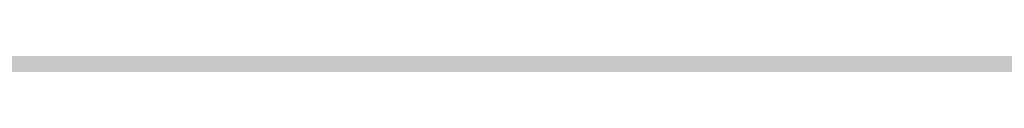
# Model space of a CAD drawing. Units: millimetres. Extents: x 0 to 2267, y 0 to 1823.
# Tile 171 of 256: x 1833.606 to 1838.83, y 1127.422 to 1127.431. Entities that reach past the tile are written whole.
import ezdxf

# ---------------------------------------------------------------- set-up
doc = ezdxf.new("R2010")
doc.units = ezdxf.units.MM
doc.header["$MEASUREMENT"] = 0
doc.layers.add('M-HATC', color=252, linetype='Continuous', lineweight=18)

msp = doc.modelspace()

# ---------------------------------------------------------------- hatches: boundary and pattern name
at = {"layer": 'M-HATC'}
h = msp.add_hatch(color=256, dxfattribs=at)
h.dxf.hatch_style = 1
h.paths.add_polyline_path([(2055.771, 1603.062), (1381.0868, 1603.062), (1381.0868, 1598.062), (2055.771, 1598.062)])
h.paths.add_polyline_path([(2055.771, 1598.062), (1381.0868, 1598.062), (1381.0868, 1593.062), (2055.771, 1593.062)])
h.paths.add_polyline_path([(2051.3074, 1536.7609), (1385.5504, 1536.7609), (1385.5504, 1526.7609), (1387.5504, 1526.7609), (1388.5366, 1525.0528), (1385.3319, 1521.2335), (1385.3319, 1521.2226), (2050.2542, 1522.7491), (2048.3212, 1525.0528), (2049.3074, 1526.7609), (2051.3074, 1526.7609)])
edge = h.paths.add_edge_path()
edge.add_arc((1847.5345, 1379.1492), 135, 222.603061, 222.890851, ccw=False)
edge.add_line((1748.1663, 1287.7656), (1683.0921, 1287.7656))
edge.add_arc((1583.7239, 1379.1492), 135, 317.109149, 317.396939, ccw=False)
edge.add_arc((1678.9686, 1290.6707), 5, 222.8909, 317.1091, ccw=False)
edge.add_arc((1774.2133, 1379.1492), 135, 222.603061, 222.890851, ccw=False)
edge.add_line((1674.8451, 1287.7656), (1609.7709, 1287.7656))
edge.add_arc((1510.4027, 1379.1492), 135, 317.109149, 317.396939, ccw=False)
edge.add_arc((1605.6474, 1290.6707), 5, 222.8909, 317.1091, ccw=False)
edge.add_arc((1700.8921, 1379.1492), 135, 222.603061, 222.890851, ccw=False)
edge.add_line((1601.5239, 1287.7656), (1536.4497, 1287.7656))
edge.add_arc((1437.0815, 1379.1492), 135, 317.109149, 317.396939, ccw=False)
edge.add_arc((1532.3262, 1290.6707), 5, 222.8909, 317.1091, ccw=False)
edge.add_arc((1627.5709, 1379.1492), 135, 222.603061, 222.890851, ccw=False)
edge.add_line((1528.2027, 1287.7656), (1505.9289, 1287.7656))
edge.add_spline(control_points=[(1505.9289, 1287.7656), (1504.2622, 1287.7656), (1504.2622, 1282.7656), (1505.9289, 1282.7656)], knot_values=[0, 0, 0, 0, 5, 5, 5, 5], degree=3, periodic=0)
edge.add_line((1505.9289, 1282.7656), (1930.9289, 1282.7656))
edge.add_spline(control_points=[(1930.9289, 1282.7656), (1932.5956, 1282.7656), (1932.5956, 1287.7656), (1930.9289, 1287.7656)], knot_values=[0, 0, 0, 0, 5, 5, 5, 5], degree=3, periodic=0)
edge.add_line((1930.9289, 1287.7656), (1903.0557, 1287.7656))
edge.add_arc((1803.6875, 1379.1492), 135, 317.109149, 317.396939, ccw=False)
edge.add_arc((1898.9322, 1290.6707), 5, 222.8909, 317.1091, ccw=False)
edge.add_arc((1994.1769, 1379.1492), 135, 222.603061, 222.890851, ccw=False)
edge.add_line((1894.8087, 1287.7656), (1829.7345, 1287.7656))
edge.add_arc((1730.3663, 1379.1492), 135, 317.109149, 317.396939, ccw=False)
edge.add_arc((1825.611, 1290.6707), 5, 222.8909, 317.1091, ccw=False)
edge.add_arc((1920.8557, 1379.1492), 135, 222.603061, 222.890851, ccw=False)
edge.add_line((1821.4875, 1287.7656), (1756.4133, 1287.7656))
edge.add_arc((1657.0451, 1379.1492), 135, 317.109149, 317.396939, ccw=False)
edge.add_arc((1752.2898, 1290.6707), 5, 222.8909, 317.1091, ccw=False)
edge = h.paths.add_edge_path()
edge.add_spline(control_points=[(1843.4289, 1227.2475), (1845.0956, 1227.2475), (1845.0956, 1232.2475), (1843.4289, 1232.2475)], knot_values=[0, 0, 0, 0, 5, 5, 5, 5], degree=3, periodic=0)
edge.add_line((1843.4289, 1232.2475), (1593.4289, 1232.2475))
edge.add_spline(control_points=[(1593.4289, 1232.2475), (1591.7622, 1232.2475), (1591.7622, 1227.2475), (1593.4289, 1227.2475)], knot_values=[0, 0, 0, 0, 5, 5, 5, 5], degree=3, periodic=0)
edge.add_line((1593.4289, 1227.2475), (1843.4289, 1227.2475))
h.paths.add_polyline_path([(1905.9289, 1127.4171), (1530.9289, 1127.4171, 0.414214), (1520.9289, 1117.4171), (1530.9289, 1117.4171), (1915.9289, 1117.4171, 0.414214)])
edge = h.paths.add_edge_path()
edge.add_arc((1397.0858, 1498.4078), 12.7299, 90.78215, 190.87871, ccw=False)
edge.add_line((1396.912, 1511.1365), (1428.0097, 1511.3488))
edge.add_line((1428.0097, 1511.3488), (1433.0097, 1511.3488))
edge.add_line((1433.0097, 1511.3488), (1434.439, 1511.3488))
edge.add_arc((1419.474, 1498.0804), 20, 41.561, 74.08211)
edge.add_line((1424.9592, 1517.3135), (1399.9351, 1517.2561))
edge.add_spline(control_points=[(1399.9307, 1517.2561), (1399.884, 1517.2131), (1399.8328, 1517.1689), (1399.7774, 1517.1236)], knot_values=[11.567499, 11.567499, 11.567499, 11.567499, 11.814249, 11.814249, 11.814249, 11.814249], degree=3, periodic=0)
edge.add_spline(control_points=[(1399.6328, 1517.0099), (1399.5831, 1516.9721), (1399.5307, 1516.9338), (1399.4759, 1516.8947)], knot_values=[11.167718, 11.167718, 11.167718, 11.167718, 11.365188, 11.365188, 11.365188, 11.365188], degree=3, periodic=0)
edge.add_spline(control_points=[(1399.3398, 1516.8001), (1399.1514, 1516.6719), (1398.9384, 1516.5377), (1398.704, 1516.3994)], knot_values=[10.376405, 10.376405, 10.376405, 10.376405, 11.00994, 11.00994, 11.00994, 11.00994], degree=3, periodic=0)
edge.add_spline(control_points=[(1398.6572, 1516.3719), (1398.5789, 1516.326), (1398.4983, 1516.2797), (1398.4155, 1516.2331)], knot_values=[10.125175, 10.125175, 10.125175, 10.125175, 10.334406, 10.334406, 10.334406, 10.334406], degree=3, periodic=0)
edge.add_spline(control_points=[(1398.2642, 1516.1487), (1398.196, 1516.1111), (1398.1263, 1516.0732), (1398.0555, 1516.0351)], knot_values=[9.832246, 9.832246, 9.832246, 9.832246, 9.999658, 9.999658, 9.999658, 9.999658], degree=3, periodic=0)
edge.add_spline(control_points=[(1397.9987, 1516.0048), (1397.7312, 1515.8621), (1397.446, 1515.7171), (1397.1466, 1515.5714)], knot_values=[9.161808, 9.161808, 9.161808, 9.161808, 9.787769, 9.787769, 9.787769, 9.787769], degree=3, periodic=0)
edge.add_spline(control_points=[(1397.1466, 1515.5714), (1396.8418, 1515.423), (1396.5222, 1515.274), (1396.1914, 1515.1262)], knot_values=[8.524455, 8.524455, 8.524455, 8.524455, 9.161808, 9.161808, 9.161808, 9.161808], degree=3, periodic=0)
edge.add_spline(control_points=[(1396.0777, 1515.0756), (1395.9854, 1515.0348), (1395.8922, 1514.994), (1395.7983, 1514.9534)], knot_values=[8.275193, 8.275193, 8.275193, 8.275193, 8.451726, 8.451726, 8.451726, 8.451726], degree=3, periodic=0)
edge.add_spline(control_points=[(1395.6018, 1514.8691), (1395.4997, 1514.8257), (1395.3968, 1514.7824), (1395.2932, 1514.7394)], knot_values=[7.962917, 7.962917, 7.962917, 7.962917, 8.152764, 8.152764, 8.152764, 8.152764], degree=3, periodic=0)
edge.add_spline(control_points=[(1395.2116, 1514.7057), (1394.8278, 1514.5475), (1394.4345, 1514.3929), (1394.0364, 1514.2442)], knot_values=[7.21254, 7.21254, 7.21254, 7.21254, 7.913148, 7.913148, 7.913148, 7.913148], degree=3, periodic=0)
edge.add_spline(control_points=[(1394.0364, 1514.2442), (1393.7076, 1514.1214), (1393.3754, 1514.0027), (1393.0427, 1513.8895)], knot_values=[6.633733, 6.633733, 6.633733, 6.633733, 7.21254, 7.21254, 7.21254, 7.21254], degree=3, periodic=0)
edge.add_spline(control_points=[(1392.8214, 1513.815), (1392.7198, 1513.7812), (1392.6181, 1513.7479), (1392.5166, 1513.7152)], knot_values=[6.328796, 6.328796, 6.328796, 6.328796, 6.505493, 6.505493, 6.505493, 6.505493], degree=3, periodic=0)
edge.add_spline(control_points=[(1392.5166, 1513.7152), (1392.3187, 1513.6515), (1392.1212, 1513.59), (1391.9244, 1513.531)], knot_values=[5.984605, 5.984605, 5.984605, 5.984605, 6.328796, 6.328796, 6.328796, 6.328796], degree=3, periodic=0)
edge.add_spline(control_points=[(1391.7915, 1513.4915), (1391.3122, 1513.3501), (1390.8384, 1513.2239), (1390.3784, 1513.1171)], knot_values=[5.066697, 5.066697, 5.066697, 5.066697, 5.907055, 5.907055, 5.907055, 5.907055], degree=3, periodic=0)
edge.add_spline(control_points=[(1390.3784, 1513.1171), (1390.1797, 1513.071), (1389.9836, 1513.0284), (1389.7907, 1512.9899)], knot_values=[4.70367, 4.70367, 4.70367, 4.70367, 5.066695, 5.066695, 5.066695, 5.066695], degree=3, periodic=0)
edge.add_spline(control_points=[(1389.422, 1512.9204), (1389.2459, 1512.8892), (1389.0729, 1512.8617), (1388.9036, 1512.8381)], knot_values=[4.130571, 4.130571, 4.130571, 4.130571, 4.469816, 4.469816, 4.469816, 4.469816], degree=3, periodic=0)
edge.add_spline(control_points=[(1388.9036, 1512.8381), (1388.591, 1512.7946), (1388.2911, 1512.7644), (1388.0071, 1512.7494)], knot_values=[3.504031, 3.504031, 3.504031, 3.504031, 4.130571, 4.130571, 4.130571, 4.130571], degree=3, periodic=0)
edge.add_spline(control_points=[(1387.9356, 1512.7459), (1387.8538, 1512.7423), (1387.7733, 1512.74), (1387.6944, 1512.739)], knot_values=[3.268866, 3.268866, 3.268866, 3.268866, 3.451164, 3.451164, 3.451164, 3.451164], degree=3, periodic=0)
edge.add_spline(control_points=[(1387.3351, 1512.7443), (1387.2076, 1512.7499), (1387.0847, 1512.7597), (1386.967, 1512.7739)], knot_values=[2.670686, 2.670686, 2.670686, 2.670686, 2.984, 2.984, 2.984, 2.984], degree=3, periodic=0)
edge.add_spline(control_points=[(1386.8327, 1512.7922), (1386.8209, 1512.7941), (1386.8092, 1512.7959), (1386.7975, 1512.7979)], knot_values=[2.516981, 2.516981, 2.516981, 2.516981, 2.549528, 2.549528, 2.549528, 2.549528], degree=3, periodic=0)
edge.add_spline(control_points=[(1386.4526, 1512.8735), (1386.4257, 1512.881), (1386.3993, 1512.889), (1386.3733, 1512.8972)], knot_values=[2.095869, 2.095869, 2.095869, 2.095869, 2.17941, 2.17941, 2.17941, 2.17941], degree=3, periodic=0)
edge.add_spline(control_points=[(1386.0691, 1513.0189), (1386.0634, 1513.0217), (1386.0577, 1513.0246), (1386.052, 1513.0275)], knot_values=[1.72453, 1.72453, 1.72453, 1.72453, 1.745933, 1.745933, 1.745933, 1.745933], degree=3, periodic=0)
edge.add_arc((1399.474, 1498.0804), 20, 131.82432, 180)
edge.add_arc((1630.3336, 1505.5484), 250.9708, 181.705176, 236.427975)
edge.add_arc((1605.3399, 1483.3044), 218.7822, 238.660829, 243.34961)
edge.add_arc((1647.0911, 1510.3592), 262.8986, 183.129836, 237.853442, ccw=False)
h.paths.add_polyline_path([(1406.5369, 1391.9644, 0.149382), (1491.5506, 1296.4418, -0.129517)], flags=17)
edge = h.paths.add_edge_path()
edge.add_arc((2037.3838, 1498.0804), 20, 0, 48.26587)
edge.add_spline(control_points=[(2050.6973, 1513.0052), (2050.6512, 1512.9847), (2050.6034, 1512.9655), (2050.5539, 1512.9477)], knot_values=[1.835652, 1.835652, 1.835652, 1.835652, 2.000781, 2.000781, 2.000781, 2.000781], degree=3, periodic=0)
edge.add_spline(control_points=[(2050.4616, 1512.9166), (2050.479, 1512.9221), (2050.4963, 1512.9277), (2050.5133, 1512.9335)], knot_values=[2.045477, 2.045477, 2.045477, 2.045477, 2.101389, 2.101389, 2.101389, 2.101389], degree=3, periodic=0)
edge.add_spline(control_points=[(2050.129, 1512.8342), (2050.1984, 1512.8473), (2050.2657, 1512.8623), (2050.3308, 1512.8792)], knot_values=[2.237629, 2.237629, 2.237629, 2.237629, 2.435841, 2.435841, 2.435841, 2.435841], degree=3, periodic=0)
edge.add_spline(control_points=[(2050.0946, 1512.8278), (2050.1061, 1512.8299), (2050.1176, 1512.832), (2050.129, 1512.8342)], knot_values=[2.435841, 2.435841, 2.435841, 2.435841, 2.468321, 2.468321, 2.468321, 2.468321], degree=3, periodic=0)
edge.add_spline(control_points=[(2049.7843, 1512.7851), (2049.8552, 1512.7922), (2049.9243, 1512.8008), (2049.9917, 1512.8109)], knot_values=[2.563852, 2.563852, 2.563852, 2.563852, 2.748541, 2.748541, 2.748541, 2.748541], degree=3, periodic=0)
edge.add_spline(control_points=[(2049.4052, 1512.7617), (2049.5364, 1512.7653), (2049.6629, 1512.773), (2049.7843, 1512.7851)], knot_values=[2.748541, 2.748541, 2.748541, 2.748541, 3.064882, 3.064882, 3.064882, 3.064882], degree=3, periodic=0)
edge.add_spline(control_points=[(2049.1698, 1512.7597), (2049.2336, 1512.7591), (2049.2965, 1512.7594), (2049.3584, 1512.7606)], knot_values=[3.102309, 3.102309, 3.102309, 3.102309, 3.2503, 3.2503, 3.2503, 3.2503], degree=3, periodic=0)
edge.add_spline(control_points=[(2048.8573, 1512.7691), (2048.9638, 1512.7638), (2049.068, 1512.7606), (2049.1698, 1512.7597)], knot_values=[3.2503, 3.2503, 3.2503, 3.2503, 3.486069, 3.486069, 3.486069, 3.486069], degree=3, periodic=0)
edge.add_spline(control_points=[(2048.6924, 1512.7789), (2048.3729, 1512.8009), (2048.0345, 1512.8411), (2047.6817, 1512.897)], knot_values=[3.606429, 3.606429, 3.606429, 3.606429, 4.2989, 4.2989, 4.2989, 4.2989], degree=3, periodic=0)
edge.add_spline(control_points=[(2047.6817, 1512.897), (2047.5458, 1512.9185), (2047.4077, 1512.9424), (2047.2678, 1512.9685)], knot_values=[4.2989, 4.2989, 4.2989, 4.2989, 4.565769, 4.565769, 4.565769, 4.565769], degree=3, periodic=0)
edge.add_spline(control_points=[(2047.2678, 1512.9685), (2047.1449, 1512.9914), (2047.0207, 1513.016), (2046.8951, 1513.0422)], knot_values=[4.565769, 4.565769, 4.565769, 4.565769, 4.799971, 4.799971, 4.799971, 4.799971], degree=3, periodic=0)
edge.add_spline(control_points=[(2046.8951, 1513.0422), (2046.5286, 1513.1188), (2046.1513, 1513.209), (2045.7676, 1513.3107)], knot_values=[4.799971, 4.799971, 4.799971, 4.799971, 5.483718, 5.483718, 5.483718, 5.483718], degree=3, periodic=0)
edge.add_spline(control_points=[(2045.7676, 1513.3107), (2045.3724, 1513.4154), (2044.9704, 1513.5322), (2044.5662, 1513.6588)], knot_values=[5.483718, 5.483718, 5.483718, 5.483718, 6.187866, 6.187866, 6.187866, 6.187866], degree=3, periodic=0)
edge.add_spline(control_points=[(2044.5662, 1513.6588), (2044.4149, 1513.7061), (2044.2633, 1513.7549), (2044.1116, 1513.8048)], knot_values=[6.187866, 6.187866, 6.187866, 6.187866, 6.451551, 6.451551, 6.451551, 6.451551], degree=3, periodic=0)
edge.add_spline(control_points=[(2044.1116, 1513.8048), (2043.9967, 1513.8427), (2043.8817, 1513.8813), (2043.7668, 1513.9205)], knot_values=[6.451551, 6.451551, 6.451551, 6.451551, 6.651434, 6.651434, 6.651434, 6.651434], degree=3, periodic=0)
edge.add_spline(control_points=[(2043.7668, 1513.9205), (2043.3716, 1514.0554), (2042.9774, 1514.1979), (2042.5886, 1514.3458)], knot_values=[6.651434, 6.651434, 6.651434, 6.651434, 7.338879, 7.338879, 7.338879, 7.338879], degree=3, periodic=0)
edge.add_spline(control_points=[(2042.5886, 1514.3458), (2042.1643, 1514.5071), (2041.7465, 1514.6749), (2041.3409, 1514.846)], knot_values=[7.338879, 7.338879, 7.338879, 7.338879, 8.089209, 8.089209, 8.089209, 8.089209], degree=3, periodic=0)
edge.add_spline(control_points=[(2041.3409, 1514.846), (2041.1028, 1514.9465), (2040.869, 1515.0481), (2040.6405, 1515.1502)], knot_values=[8.089209, 8.089209, 8.089209, 8.089209, 8.529587, 8.529587, 8.529587, 8.529587], degree=3, periodic=0)
edge.add_spline(control_points=[(2040.51, 1515.2089), (2040.0824, 1515.4022), (2039.6747, 1515.5971), (2039.295, 1515.7894)], knot_values=[8.613818, 8.613818, 8.613818, 8.613818, 9.44571, 9.44571, 9.44571, 9.44571], degree=3, periodic=0)
edge.add_spline(control_points=[(2039.295, 1515.7894), (2039.0618, 1515.9075), (2038.8391, 1516.0246), (2038.6288, 1516.1398)], knot_values=[9.44571, 9.44571, 9.44571, 9.44571, 9.956404, 9.956404, 9.956404, 9.956404], degree=3, periodic=0)
edge.add_spline(control_points=[(2038.6288, 1516.1398), (2038.5187, 1516.2001), (2038.4121, 1516.2598), (2038.309, 1516.3189)], knot_values=[9.956404, 9.956404, 9.956404, 9.956404, 10.223542, 10.223542, 10.223542, 10.223542], degree=3, periodic=0)
edge.add_spline(control_points=[(2038.309, 1516.3189), (2038.2138, 1516.3735), (2038.1216, 1516.4276), (2038.0328, 1516.481)], knot_values=[10.223542, 10.223542, 10.223542, 10.223542, 10.47051, 10.47051, 10.47051, 10.47051], degree=3, periodic=0)
edge.add_spline(control_points=[(2038.0328, 1516.481), (2037.7855, 1516.6296), (2037.5639, 1516.773), (2037.3722, 1516.909)], knot_values=[10.47051, 10.47051, 10.47051, 10.47051, 11.15767, 11.15767, 11.15767, 11.15767], degree=3, periodic=0)
edge.add_spline(control_points=[(2037.3722, 1516.909), (2037.2789, 1516.9752), (2037.1927, 1517.0396), (2037.1142, 1517.102)], knot_values=[11.15767, 11.15767, 11.15767, 11.15767, 11.49227, 11.49227, 11.49227, 11.49227], degree=3, periodic=0)
edge.add_spline(control_points=[(2036.8564, 1517.3259), (2036.9148, 1517.2692), (2036.9814, 1517.2103), (2037.0557, 1517.1492)], knot_values=[11.577341, 11.577341, 11.577341, 11.577341, 11.91035, 11.91035, 11.91035, 11.91035], degree=3, periodic=0)
edge.add_spline(control_points=[(2036.8074, 1517.3748), (2036.823, 1517.3587), (2036.8393, 1517.3424), (2036.8564, 1517.3259)], knot_values=[11.91035, 11.91035, 11.91035, 11.91035, 12.007402, 12.007402, 12.007402, 12.007402], degree=3, periodic=0)
edge.add_spline(control_points=[(2036.7017, 1517.494), (2036.7104, 1517.483), (2036.7196, 1517.4719), (2036.7291, 1517.4606)], knot_values=[12.184155, 12.184155, 12.184155, 12.184155, 12.255409, 12.255409, 12.255409, 12.255409], degree=3, periodic=0)
edge.add_spline(control_points=[(2036.6159, 1517.6205), (2036.62, 1517.613), (2036.6243, 1517.6055), (2036.6289, 1517.5979)], knot_values=[12.487913, 12.487913, 12.487913, 12.487913, 12.541035, 12.541035, 12.541035, 12.541035], degree=3, periodic=0)
edge.add_spline(control_points=[(2036.5635, 1517.786), (2036.5637, 1517.7794), (2036.5642, 1517.7726), (2036.565, 1517.7658)], knot_values=[12.911761, 12.911761, 12.911761, 12.911761, 12.968286, 12.968286, 12.968286, 12.968286], degree=3, periodic=0)
edge.add_spline(control_points=[(2036.6166, 1517.9304), (2036.6125, 1517.9259), (2036.6086, 1517.9212), (2036.6049, 1517.9165)], knot_values=[13.382527, 13.382527, 13.382527, 13.382527, 13.433791, 13.433791, 13.433791, 13.433791], degree=3, periodic=0)
edge.add_spline(control_points=[(2036.749, 1518.017), (2036.7361, 1518.0116), (2036.7239, 1518.006), (2036.7124, 1518.0002)], knot_values=[13.726299, 13.726299, 13.726299, 13.726299, 13.809928, 13.809928, 13.809928, 13.809928], degree=3, periodic=0)
edge.add_spline(control_points=[(2036.8604, 1518.0528), (2036.8386, 1518.0474), (2036.8181, 1518.0416), (2036.7988, 1518.0353)], knot_values=[13.910887, 13.910887, 13.910887, 13.910887, 14.02153, 14.02153, 14.02153, 14.02153], degree=3, periodic=0)
edge.add_line((2036.9639, 1518.0804), (2032.3838, 1518.0804))
edge.add_line((2032.3838, 1518.0804), (2027.3838, 1518.0804))
edge.add_line((2027.3838, 1518.0804), (2022.3838, 1518.0804))
edge.add_line((2022.3838, 1518.0804), (2017.3838, 1518.0804))
edge.add_arc((2017.3838, 1498.0804), 20, 90, 138.439)
edge.add_line((2002.4188, 1511.3488), (2003.8481, 1511.3488))
edge.add_line((2003.8481, 1511.3488), (2008.8481, 1511.3488))
edge.add_line((2008.8481, 1511.3488), (2039.772, 1511.1377))
edge.add_arc((2039.772, 1498.4078), 12.7299, -10.87871, 90, ccw=False)
edge.add_arc((1789.7668, 1510.3592), 262.8986, 302.146558, 356.870164, ccw=False)
edge.add_arc((1831.5179, 1483.3044), 218.7822, 296.65039, 301.339171)
edge.add_arc((1806.5242, 1505.5484), 250.9708, 303.572025, 358.294824)
h.paths.add_polyline_path([(2030.321, 1391.9644, -0.129517), (1945.3072, 1296.4418, 0.149382)], flags=17)
edge = h.paths.add_edge_path()
edge.add_spline(control_points=[(2037.2464, 1518.0821), (2037.2898, 1518.081), (2037.3355, 1518.0804), (2037.3838, 1518.0804)], knot_values=[0.000012, 0.000012, 0.000012, 0.000012, 0.144754, 0.144754, 0.144754, 0.144754], degree=3, periodic=0)
edge.add_line((2037.3357, 1518.0804), (2037.0096, 1518.0804))
edge.add_spline(control_points=[(2037.0096, 1518.0804), (2036.9822, 1518.0768), (2036.956, 1518.0727), (2036.9312, 1518.0681)], knot_values=[14.13465, 14.13465, 14.13465, 14.13465, 14.247197, 14.247197, 14.247197, 14.247197], degree=3, periodic=0)
edge.add_spline(control_points=[(2036.9312, 1518.0681), (2036.9276, 1518.0674), (2036.9241, 1518.0667), (2036.9205, 1518.0661)], knot_values=[14.118315, 14.118315, 14.118315, 14.118315, 14.13465, 14.13465, 14.13465, 14.13465], degree=3, periodic=0)
edge.add_spline(control_points=[(2036.9205, 1518.0661), (2036.9118, 1518.0644), (2036.9032, 1518.0626), (2036.8948, 1518.0608)], knot_values=[14.078086, 14.078086, 14.078086, 14.078086, 14.118315, 14.118315, 14.118315, 14.118315], degree=3, periodic=0)
edge.add_spline(control_points=[(2036.8948, 1518.0608), (2036.883, 1518.0583), (2036.8716, 1518.0556), (2036.8604, 1518.0528)], knot_values=[14.02153, 14.02153, 14.02153, 14.02153, 14.078086, 14.078086, 14.078086, 14.078086], degree=3, periodic=0)
edge.add_spline(control_points=[(2036.8604, 1518.0528), (2036.8386, 1518.0474), (2036.8181, 1518.0416), (2036.7988, 1518.0353)], knot_values=[13.910887, 13.910887, 13.910887, 13.910887, 14.02153, 14.02153, 14.02153, 14.02153], degree=3, periodic=0)
edge.add_spline(control_points=[(2036.7988, 1518.0353), (2036.7981, 1518.035), (2036.7974, 1518.0348), (2036.7967, 1518.0346)], knot_values=[13.906906, 13.906906, 13.906906, 13.906906, 13.910887, 13.910887, 13.910887, 13.910887], degree=3, periodic=0)
edge.add_spline(control_points=[(2036.7967, 1518.0346), (2036.7882, 1518.0318), (2036.7799, 1518.0289), (2036.7719, 1518.0259)], knot_values=[13.857826, 13.857826, 13.857826, 13.857826, 13.906906, 13.906906, 13.906906, 13.906906], degree=3, periodic=0)
edge.add_spline(control_points=[(2036.7719, 1518.0259), (2036.764, 1518.023), (2036.7564, 1518.02), (2036.749, 1518.017)], knot_values=[13.809928, 13.809928, 13.809928, 13.809928, 13.857826, 13.857826, 13.857826, 13.857826], degree=3, periodic=0)
edge.add_spline(control_points=[(2036.749, 1518.017), (2036.7361, 1518.0116), (2036.7239, 1518.006), (2036.7124, 1518.0002)], knot_values=[13.726299, 13.726299, 13.726299, 13.726299, 13.809928, 13.809928, 13.809928, 13.809928], degree=3, periodic=0)
edge.add_spline(control_points=[(2036.7124, 1518.0002), (2036.7121, 1518), (2036.7118, 1517.9999), (2036.7115, 1517.9997)], knot_values=[13.723993, 13.723993, 13.723993, 13.723993, 13.726299, 13.726299, 13.726299, 13.726299], degree=3, periodic=0)
edge.add_spline(control_points=[(2036.7115, 1517.9997), (2036.7063, 1517.9971), (2036.7013, 1517.9944), (2036.6965, 1517.9917)], knot_values=[13.686536, 13.686536, 13.686536, 13.686536, 13.723993, 13.723993, 13.723993, 13.723993], degree=3, periodic=0)
edge.add_spline(control_points=[(2036.6965, 1517.9917), (2036.6919, 1517.9891), (2036.6874, 1517.9865), (2036.6831, 1517.9839)], knot_values=[13.651251, 13.651251, 13.651251, 13.651251, 13.686536, 13.686536, 13.686536, 13.686536], degree=3, periodic=0)
edge.add_spline(control_points=[(2036.6831, 1517.9839), (2036.6764, 1517.9798), (2036.67, 1517.9757), (2036.6639, 1517.9714)], knot_values=[13.596804, 13.596804, 13.596804, 13.596804, 13.651251, 13.651251, 13.651251, 13.651251], degree=3, periodic=0)
edge.add_spline(control_points=[(2036.6639, 1517.9714), (2036.6636, 1517.9712), (2036.6633, 1517.9709), (2036.6629, 1517.9707)], knot_values=[13.593956, 13.593956, 13.593956, 13.593956, 13.596804, 13.596804, 13.596804, 13.596804], degree=3, periodic=0)
edge.add_spline(control_points=[(2036.6629, 1517.9707), (2036.6603, 1517.9689), (2036.6577, 1517.967), (2036.6552, 1517.9651)], knot_values=[13.570322, 13.570322, 13.570322, 13.570322, 13.593956, 13.593956, 13.593956, 13.593956], degree=3, periodic=0)
edge.add_spline(control_points=[(2036.6552, 1517.9651), (2036.6525, 1517.9631), (2036.6499, 1517.9611), (2036.6474, 1517.9591)], knot_values=[13.545477, 13.545477, 13.545477, 13.545477, 13.570322, 13.570322, 13.570322, 13.570322], degree=3, periodic=0)
edge.add_spline(control_points=[(2036.6474, 1517.9591), (2036.6472, 1517.9589), (2036.6471, 1517.9588), (2036.6469, 1517.9587)], knot_values=[13.543931, 13.543931, 13.543931, 13.543931, 13.545477, 13.545477, 13.545477, 13.545477], degree=3, periodic=0)
edge.add_spline(control_points=[(2036.6469, 1517.9587), (2036.6412, 1517.9541), (2036.6358, 1517.9494), (2036.6307, 1517.9447)], knot_values=[13.488237, 13.488237, 13.488237, 13.488237, 13.543931, 13.543931, 13.543931, 13.543931], degree=3, periodic=0)
edge.add_spline(control_points=[(2036.6307, 1517.9447), (2036.6282, 1517.9423), (2036.6257, 1517.9399), (2036.6233, 1517.9374)], knot_values=[13.460307, 13.460307, 13.460307, 13.460307, 13.488237, 13.488237, 13.488237, 13.488237], degree=3, periodic=0)
edge.add_spline(control_points=[(2036.6233, 1517.9374), (2036.6215, 1517.9356), (2036.6198, 1517.9338), (2036.6181, 1517.932)], knot_values=[13.439712, 13.439712, 13.439712, 13.439712, 13.460307, 13.460307, 13.460307, 13.460307], degree=3, periodic=0)
edge.add_spline(control_points=[(2036.6181, 1517.932), (2036.6176, 1517.9315), (2036.6171, 1517.9309), (2036.6166, 1517.9304)], knot_values=[13.433791, 13.433791, 13.433791, 13.433791, 13.439712, 13.439712, 13.439712, 13.439712], degree=3, periodic=0)
edge.add_spline(control_points=[(2036.6166, 1517.9304), (2036.6125, 1517.9259), (2036.6086, 1517.9212), (2036.6049, 1517.9165)], knot_values=[13.382527, 13.382527, 13.382527, 13.382527, 13.433791, 13.433791, 13.433791, 13.433791], degree=3, periodic=0)
edge.add_spline(control_points=[(2036.6049, 1517.9165), (2036.6026, 1517.9135), (2036.6004, 1517.9104), (2036.5982, 1517.9074)], knot_values=[13.350017, 13.350017, 13.350017, 13.350017, 13.382527, 13.382527, 13.382527, 13.382527], degree=3, periodic=0)
edge.add_spline(control_points=[(2036.5982, 1517.9074), (2036.5972, 1517.9059), (2036.5962, 1517.9043), (2036.5952, 1517.9028)], knot_values=[13.333922, 13.333922, 13.333922, 13.333922, 13.350017, 13.350017, 13.350017, 13.350017], degree=3, periodic=0)
edge.add_spline(control_points=[(2036.5952, 1517.9028), (2036.5945, 1517.9018), (2036.5939, 1517.9009), (2036.5933, 1517.8999)], knot_values=[13.323828, 13.323828, 13.323828, 13.323828, 13.333922, 13.333922, 13.333922, 13.333922], degree=3, periodic=0)
edge.add_spline(control_points=[(2036.5933, 1517.8999), (2036.5905, 1517.8955), (2036.5879, 1517.8909), (2036.5855, 1517.8864)], knot_values=[13.277545, 13.277545, 13.277545, 13.277545, 13.323828, 13.323828, 13.323828, 13.323828], degree=3, periodic=0)
edge.add_spline(control_points=[(2036.5855, 1517.8864), (2036.5836, 1517.8827), (2036.5817, 1517.8789), (2036.5801, 1517.8751)], knot_values=[13.240119, 13.240119, 13.240119, 13.240119, 13.277545, 13.277545, 13.277545, 13.277545], degree=3, periodic=0)
edge.add_spline(control_points=[(2036.5801, 1517.8751), (2036.5795, 1517.8739), (2036.579, 1517.8727), (2036.5785, 1517.8715)], knot_values=[13.228211, 13.228211, 13.228211, 13.228211, 13.240119, 13.240119, 13.240119, 13.240119], degree=3, periodic=0)
edge.add_spline(control_points=[(2036.5785, 1517.8715), (2036.578, 1517.8702), (2036.5774, 1517.869), (2036.5769, 1517.8677)], knot_values=[13.215717, 13.215717, 13.215717, 13.215717, 13.228211, 13.228211, 13.228211, 13.228211], degree=3, periodic=0)
edge.add_spline(control_points=[(2036.5769, 1517.8677), (2036.5755, 1517.864), (2036.5741, 1517.8603), (2036.5729, 1517.8565)], knot_values=[13.179847, 13.179847, 13.179847, 13.179847, 13.215717, 13.215717, 13.215717, 13.215717], degree=3, periodic=0)
edge.add_spline(control_points=[(2036.5729, 1517.8565), (2036.5713, 1517.8515), (2036.5699, 1517.8464), (2036.5687, 1517.8413)], knot_values=[13.132017, 13.132017, 13.132017, 13.132017, 13.179847, 13.179847, 13.179847, 13.179847], degree=3, periodic=0)
edge.add_spline(control_points=[(2036.5687, 1517.8413), (2036.5684, 1517.8402), (2036.5682, 1517.8392), (2036.568, 1517.8382)], knot_values=[13.122482, 13.122482, 13.122482, 13.122482, 13.132017, 13.132017, 13.132017, 13.132017], degree=3, periodic=0)
edge.add_spline(control_points=[(2036.568, 1517.8382), (2036.5676, 1517.8363), (2036.5672, 1517.8345), (2036.5669, 1517.8327)], knot_values=[13.105592, 13.105592, 13.105592, 13.105592, 13.122482, 13.122482, 13.122482, 13.122482], degree=3, periodic=0)
edge.add_spline(control_points=[(2036.5669, 1517.8327), (2036.5662, 1517.8292), (2036.5657, 1517.8257), (2036.5652, 1517.8222)], knot_values=[13.074063, 13.074063, 13.074063, 13.074063, 13.105592, 13.105592, 13.105592, 13.105592], degree=3, periodic=0)
edge.add_spline(control_points=[(2036.5652, 1517.8222), (2036.5652, 1517.8222), (2036.5652, 1517.8222), (2036.5652, 1517.8222)], knot_values=[13.074043, 13.074043, 13.074043, 13.074043, 13.074063, 13.074063, 13.074063, 13.074063], degree=3, periodic=0)
edge.add_spline(control_points=[(2036.5652, 1517.8222), (2036.5644, 1517.8164), (2036.5639, 1517.8106), (2036.5636, 1517.8046)], knot_values=[13.021884, 13.021884, 13.021884, 13.021884, 13.074043, 13.074043, 13.074043, 13.074043], degree=3, periodic=0)
edge.add_spline(control_points=[(2036.5636, 1517.8046), (2036.5636, 1517.804), (2036.5636, 1517.8034), (2036.5635, 1517.8028)], knot_values=[13.01674, 13.01674, 13.01674, 13.01674, 13.021884, 13.021884, 13.021884, 13.021884], degree=3, periodic=0)
edge.add_spline(control_points=[(2036.5635, 1517.8028), (2036.5634, 1517.8005), (2036.5634, 1517.7982), (2036.5634, 1517.7958)], knot_values=[12.996438, 12.996438, 12.996438, 12.996438, 13.01674, 13.01674, 13.01674, 13.01674], degree=3, periodic=0)
edge.add_spline(control_points=[(2036.5634, 1517.7958), (2036.5633, 1517.7926), (2036.5634, 1517.7893), (2036.5635, 1517.786)], knot_values=[12.968286, 12.968286, 12.968286, 12.968286, 12.996438, 12.996438, 12.996438, 12.996438], degree=3, periodic=0)
edge.add_spline(control_points=[(2036.5635, 1517.786), (2036.5637, 1517.7794), (2036.5642, 1517.7726), (2036.565, 1517.7658)], knot_values=[12.911761, 12.911761, 12.911761, 12.911761, 12.968286, 12.968286, 12.968286, 12.968286], degree=3, periodic=0)
edge.add_spline(control_points=[(2036.565, 1517.7658), (2036.565, 1517.7657), (2036.565, 1517.7656), (2036.565, 1517.7656)], knot_values=[12.911017, 12.911017, 12.911017, 12.911017, 12.911761, 12.911761, 12.911761, 12.911761], degree=3, periodic=0)
edge.add_spline(control_points=[(2036.565, 1517.7656), (2036.5654, 1517.7625), (2036.5658, 1517.7593), (2036.5663, 1517.7562)], knot_values=[12.88528, 12.88528, 12.88528, 12.88528, 12.911017, 12.911017, 12.911017, 12.911017], degree=3, periodic=0)
edge.add_spline(control_points=[(2036.5663, 1517.7562), (2036.5667, 1517.7534), (2036.5672, 1517.7506), (2036.5677, 1517.7478)], knot_values=[12.862519, 12.862519, 12.862519, 12.862519, 12.88528, 12.88528, 12.88528, 12.88528], degree=3, periodic=0)
edge.add_spline(control_points=[(2036.5677, 1517.7478), (2036.5678, 1517.7474), (2036.5679, 1517.7469), (2036.568, 1517.7465)], knot_values=[12.858885, 12.858885, 12.858885, 12.858885, 12.862519, 12.862519, 12.862519, 12.862519], degree=3, periodic=0)
edge.add_spline(control_points=[(2036.568, 1517.7465), (2036.5692, 1517.7399), (2036.5707, 1517.7332), (2036.5724, 1517.7264)], knot_values=[12.8053, 12.8053, 12.8053, 12.8053, 12.858885, 12.858885, 12.858885, 12.858885], degree=3, periodic=0)
edge.add_spline(control_points=[(2036.5724, 1517.7264), (2036.5734, 1517.7226), (2036.5745, 1517.7187), (2036.5756, 1517.7149)], knot_values=[12.775176, 12.775176, 12.775176, 12.775176, 12.8053, 12.8053, 12.8053, 12.8053], degree=3, periodic=0)
edge.add_spline(control_points=[(2036.5756, 1517.7149), (2036.5763, 1517.7125), (2036.577, 1517.7102), (2036.5778, 1517.7078)], knot_values=[12.756759, 12.756759, 12.756759, 12.756759, 12.775176, 12.775176, 12.775176, 12.775176], degree=3, periodic=0)
edge.add_spline(control_points=[(2036.5778, 1517.7078), (2036.5781, 1517.7067), (2036.5784, 1517.7057), (2036.5787, 1517.7047)], knot_values=[12.748742, 12.748742, 12.748742, 12.748742, 12.756759, 12.756759, 12.756759, 12.756759], degree=3, periodic=0)
edge.add_spline(control_points=[(2036.5787, 1517.7047), (2036.5808, 1517.6983), (2036.5831, 1517.6919), (2036.5856, 1517.6854)], knot_values=[12.69959, 12.69959, 12.69959, 12.69959, 12.748742, 12.748742, 12.748742, 12.748742], degree=3, periodic=0)
edge.add_spline(control_points=[(2036.5856, 1517.6854), (2036.5876, 1517.68), (2036.5898, 1517.6746), (2036.5921, 1517.6692)], knot_values=[12.659038, 12.659038, 12.659038, 12.659038, 12.69959, 12.69959, 12.69959, 12.69959], degree=3, periodic=0)
edge.add_spline(control_points=[(2036.5921, 1517.6692), (2036.594, 1517.6648), (2036.5959, 1517.6605), (2036.5979, 1517.6561)], knot_values=[12.626806, 12.626806, 12.626806, 12.626806, 12.659038, 12.659038, 12.659038, 12.659038], degree=3, periodic=0)
edge.add_spline(control_points=[(2036.5979, 1517.6561), (2036.5984, 1517.6551), (2036.5989, 1517.6541), (2036.5993, 1517.6531)], knot_values=[12.619394, 12.619394, 12.619394, 12.619394, 12.626806, 12.626806, 12.626806, 12.626806], degree=3, periodic=0)
edge.add_spline(control_points=[(2036.5993, 1517.6531), (2036.6043, 1517.6424), (2036.6099, 1517.6315), (2036.6159, 1517.6205)], knot_values=[12.541039, 12.541039, 12.541039, 12.541039, 12.619394, 12.619394, 12.619394, 12.619394], degree=3, periodic=0)
edge.add_spline(control_points=[(2036.6159, 1517.6205), (2036.6159, 1517.6205), (2036.6159, 1517.6205), (2036.6159, 1517.6205)], knot_values=[12.541035, 12.541035, 12.541035, 12.541035, 12.541039, 12.541039, 12.541039, 12.541039], degree=3, periodic=0)
edge.add_spline(control_points=[(2036.6159, 1517.6205), (2036.62, 1517.613), (2036.6243, 1517.6055), (2036.6289, 1517.5979)], knot_values=[12.487913, 12.487913, 12.487913, 12.487913, 12.541035, 12.541035, 12.541035, 12.541035], degree=3, periodic=0)
edge.add_spline(control_points=[(2036.6289, 1517.5979), (2036.6326, 1517.5916), (2036.6365, 1517.5853), (2036.6406, 1517.5789)], knot_values=[12.443982, 12.443982, 12.443982, 12.443982, 12.487913, 12.487913, 12.487913, 12.487913], degree=3, periodic=0)
edge.add_spline(control_points=[(2036.6406, 1517.5789), (2036.6414, 1517.5776), (2036.6423, 1517.5763), (2036.6431, 1517.5749)], knot_values=[12.434996, 12.434996, 12.434996, 12.434996, 12.443982, 12.443982, 12.443982, 12.443982], degree=3, periodic=0)
edge.add_spline(control_points=[(2036.6431, 1517.5749), (2036.6531, 1517.5596), (2036.6639, 1517.5439), (2036.6756, 1517.528)], knot_values=[12.329647, 12.329647, 12.329647, 12.329647, 12.434996, 12.434996, 12.434996, 12.434996], degree=3, periodic=0)
edge.add_spline(control_points=[(2036.6756, 1517.528), (2036.6839, 1517.5168), (2036.6925, 1517.5055), (2036.7017, 1517.494)], knot_values=[12.255409, 12.255409, 12.255409, 12.255409, 12.329647, 12.329647, 12.329647, 12.329647], degree=3, periodic=0)
edge.add_spline(control_points=[(2036.7017, 1517.494), (2036.7104, 1517.483), (2036.7196, 1517.4719), (2036.7291, 1517.4606)], knot_values=[12.184155, 12.184155, 12.184155, 12.184155, 12.255409, 12.255409, 12.255409, 12.255409], degree=3, periodic=0)
edge.add_spline(control_points=[(2036.7291, 1517.4606), (2036.7436, 1517.4435), (2036.759, 1517.4262), (2036.7753, 1517.4085)], knot_values=[12.075961, 12.075961, 12.075961, 12.075961, 12.184155, 12.184155, 12.184155, 12.184155], degree=3, periodic=0)
edge.add_spline(control_points=[(2036.7753, 1517.4085), (2036.7763, 1517.4075), (2036.7773, 1517.4064), (2036.7783, 1517.4054)], knot_values=[12.069502, 12.069502, 12.069502, 12.069502, 12.075961, 12.075961, 12.075961, 12.075961], degree=3, periodic=0)
edge.add_spline(control_points=[(2036.7783, 1517.4054), (2036.7877, 1517.3953), (2036.7974, 1517.385), (2036.8074, 1517.3748)], knot_values=[12.007402, 12.007402, 12.007402, 12.007402, 12.069502, 12.069502, 12.069502, 12.069502], degree=3, periodic=0)
edge.add_spline(control_points=[(2036.8074, 1517.3748), (2036.823, 1517.3587), (2036.8393, 1517.3424), (2036.8564, 1517.3259)], knot_values=[11.91035, 11.91035, 11.91035, 11.91035, 12.007402, 12.007402, 12.007402, 12.007402], degree=3, periodic=0)
edge.add_spline(control_points=[(2036.8564, 1517.3259), (2036.9148, 1517.2692), (2036.9814, 1517.2103), (2037.0557, 1517.1492)], knot_values=[11.577341, 11.577341, 11.577341, 11.577341, 11.91035, 11.91035, 11.91035, 11.91035], degree=3, periodic=0)
edge.add_spline(control_points=[(2037.0557, 1517.1492), (2037.0747, 1517.1336), (2037.0942, 1517.1179), (2037.1142, 1517.102)], knot_values=[11.49227, 11.49227, 11.49227, 11.49227, 11.577341, 11.577341, 11.577341, 11.577341], degree=3, periodic=0)
edge.add_spline(control_points=[(2037.1142, 1517.102), (2037.1927, 1517.0396), (2037.2789, 1516.9752), (2037.3722, 1516.909)], knot_values=[11.15767, 11.15767, 11.15767, 11.15767, 11.49227, 11.49227, 11.49227, 11.49227], degree=3, periodic=0)
edge.add_spline(control_points=[(2037.3722, 1516.909), (2037.5639, 1516.773), (2037.7855, 1516.6296), (2038.0328, 1516.481)], knot_values=[10.47051, 10.47051, 10.47051, 10.47051, 11.15767, 11.15767, 11.15767, 11.15767], degree=3, periodic=0)
edge.add_spline(control_points=[(2038.0328, 1516.481), (2038.1216, 1516.4276), (2038.2138, 1516.3735), (2038.309, 1516.3189)], knot_values=[10.223542, 10.223542, 10.223542, 10.223542, 10.47051, 10.47051, 10.47051, 10.47051], degree=3, periodic=0)
edge.add_spline(control_points=[(2038.309, 1516.3189), (2038.4121, 1516.2598), (2038.5187, 1516.2001), (2038.6288, 1516.1398)], knot_values=[9.956404, 9.956404, 9.956404, 9.956404, 10.223542, 10.223542, 10.223542, 10.223542], degree=3, periodic=0)
edge.add_spline(control_points=[(2038.6288, 1516.1398), (2038.8391, 1516.0246), (2039.0618, 1515.9075), (2039.295, 1515.7894)], knot_values=[9.44571, 9.44571, 9.44571, 9.44571, 9.956404, 9.956404, 9.956404, 9.956404], degree=3, periodic=0)
edge.add_spline(control_points=[(2039.295, 1515.7894), (2039.6747, 1515.5971), (2040.0824, 1515.4022), (2040.51, 1515.2089)], knot_values=[8.613818, 8.613818, 8.613818, 8.613818, 9.44571, 9.44571, 9.44571, 9.44571], degree=3, periodic=0)
edge.add_spline(control_points=[(2040.51, 1515.2089), (2040.5533, 1515.1893), (2040.5968, 1515.1697), (2040.6405, 1515.1502)], knot_values=[8.529587, 8.529587, 8.529587, 8.529587, 8.613818, 8.613818, 8.613818, 8.613818], degree=3, periodic=0)
edge.add_spline(control_points=[(2040.6405, 1515.1502), (2040.869, 1515.0481), (2041.1028, 1514.9465), (2041.3409, 1514.846)], knot_values=[8.089209, 8.089209, 8.089209, 8.089209, 8.529587, 8.529587, 8.529587, 8.529587], degree=3, periodic=0)
edge.add_spline(control_points=[(2041.3409, 1514.846), (2041.7465, 1514.6749), (2042.1643, 1514.5071), (2042.5886, 1514.3458)], knot_values=[7.338879, 7.338879, 7.338879, 7.338879, 8.089209, 8.089209, 8.089209, 8.089209], degree=3, periodic=0)
edge.add_spline(control_points=[(2042.5886, 1514.3458), (2042.9774, 1514.1979), (2043.3716, 1514.0554), (2043.7668, 1513.9205)], knot_values=[6.651434, 6.651434, 6.651434, 6.651434, 7.338879, 7.338879, 7.338879, 7.338879], degree=3, periodic=0)
edge.add_spline(control_points=[(2043.7668, 1513.9205), (2043.8817, 1513.8813), (2043.9967, 1513.8427), (2044.1116, 1513.8048)], knot_values=[6.451551, 6.451551, 6.451551, 6.451551, 6.651434, 6.651434, 6.651434, 6.651434], degree=3, periodic=0)
edge.add_spline(control_points=[(2044.1116, 1513.8048), (2044.2633, 1513.7549), (2044.4149, 1513.7061), (2044.5662, 1513.6588)], knot_values=[6.187866, 6.187866, 6.187866, 6.187866, 6.451551, 6.451551, 6.451551, 6.451551], degree=3, periodic=0)
edge.add_spline(control_points=[(2044.5662, 1513.6588), (2044.9704, 1513.5322), (2045.3724, 1513.4154), (2045.7676, 1513.3107)], knot_values=[5.483718, 5.483718, 5.483718, 5.483718, 6.187866, 6.187866, 6.187866, 6.187866], degree=3, periodic=0)
edge.add_spline(control_points=[(2045.7676, 1513.3107), (2046.1513, 1513.209), (2046.5286, 1513.1188), (2046.8951, 1513.0422)], knot_values=[4.799971, 4.799971, 4.799971, 4.799971, 5.483718, 5.483718, 5.483718, 5.483718], degree=3, periodic=0)
edge.add_spline(control_points=[(2046.8951, 1513.0422), (2047.0207, 1513.016), (2047.1449, 1512.9914), (2047.2678, 1512.9685)], knot_values=[4.565769, 4.565769, 4.565769, 4.565769, 4.799971, 4.799971, 4.799971, 4.799971], degree=3, periodic=0)
edge.add_spline(control_points=[(2047.2678, 1512.9685), (2047.4077, 1512.9424), (2047.5458, 1512.9185), (2047.6817, 1512.897)], knot_values=[4.2989, 4.2989, 4.2989, 4.2989, 4.565769, 4.565769, 4.565769, 4.565769], degree=3, periodic=0)
edge.add_spline(control_points=[(2047.6817, 1512.897), (2048.0345, 1512.8411), (2048.3729, 1512.8009), (2048.6924, 1512.7789)], knot_values=[3.606429, 3.606429, 3.606429, 3.606429, 4.2989, 4.2989, 4.2989, 4.2989], degree=3, periodic=0)
edge.add_spline(control_points=[(2048.6924, 1512.7789), (2048.7479, 1512.7751), (2048.8029, 1512.7718), (2048.8573, 1512.7691)], knot_values=[3.486069, 3.486069, 3.486069, 3.486069, 3.606429, 3.606429, 3.606429, 3.606429], degree=3, periodic=0)
edge.add_spline(control_points=[(2048.8573, 1512.7691), (2048.9638, 1512.7638), (2049.068, 1512.7606), (2049.1698, 1512.7597)], knot_values=[3.2503, 3.2503, 3.2503, 3.2503, 3.486069, 3.486069, 3.486069, 3.486069], degree=3, periodic=0)
edge.add_spline(control_points=[(2049.1698, 1512.7597), (2049.2336, 1512.7591), (2049.2965, 1512.7594), (2049.3584, 1512.7606)], knot_values=[3.102309, 3.102309, 3.102309, 3.102309, 3.2503, 3.2503, 3.2503, 3.2503], degree=3, periodic=0)
edge.add_spline(control_points=[(2049.3584, 1512.7606), (2049.3741, 1512.7609), (2049.3897, 1512.7613), (2049.4052, 1512.7617)], knot_values=[3.064882, 3.064882, 3.064882, 3.064882, 3.102309, 3.102309, 3.102309, 3.102309], degree=3, periodic=0)
edge.add_spline(control_points=[(2049.4052, 1512.7617), (2049.5364, 1512.7653), (2049.6629, 1512.773), (2049.7843, 1512.7851)], knot_values=[2.748541, 2.748541, 2.748541, 2.748541, 3.064882, 3.064882, 3.064882, 3.064882], degree=3, periodic=0)
edge.add_spline(control_points=[(2049.7843, 1512.7851), (2049.8552, 1512.7922), (2049.9243, 1512.8008), (2049.9917, 1512.8109)], knot_values=[2.563852, 2.563852, 2.563852, 2.563852, 2.748541, 2.748541, 2.748541, 2.748541], degree=3, periodic=0)
edge.add_spline(control_points=[(2049.9917, 1512.8109), (2050.0265, 1512.8161), (2050.0608, 1512.8218), (2050.0946, 1512.8278)], knot_values=[2.468321, 2.468321, 2.468321, 2.468321, 2.563852, 2.563852, 2.563852, 2.563852], degree=3, periodic=0)
edge.add_spline(control_points=[(2050.0946, 1512.8278), (2050.1061, 1512.8299), (2050.1176, 1512.832), (2050.129, 1512.8342)], knot_values=[2.435841, 2.435841, 2.435841, 2.435841, 2.468321, 2.468321, 2.468321, 2.468321], degree=3, periodic=0)
edge.add_spline(control_points=[(2050.129, 1512.8342), (2050.1984, 1512.8473), (2050.2657, 1512.8623), (2050.3308, 1512.8792)], knot_values=[2.237629, 2.237629, 2.237629, 2.237629, 2.435841, 2.435841, 2.435841, 2.435841], degree=3, periodic=0)
edge.add_spline(control_points=[(2050.3308, 1512.8792), (2050.3754, 1512.8908), (2050.4191, 1512.9032), (2050.4616, 1512.9166)], knot_values=[2.101389, 2.101389, 2.101389, 2.101389, 2.237629, 2.237629, 2.237629, 2.237629], degree=3, periodic=0)
edge.add_spline(control_points=[(2050.4616, 1512.9166), (2050.479, 1512.9221), (2050.4963, 1512.9277), (2050.5133, 1512.9335)], knot_values=[2.045477, 2.045477, 2.045477, 2.045477, 2.101389, 2.101389, 2.101389, 2.101389], degree=3, periodic=0)
edge.add_spline(control_points=[(2050.5133, 1512.9335), (2050.527, 1512.9382), (2050.5405, 1512.9429), (2050.5539, 1512.9477)], knot_values=[2.000781, 2.000781, 2.000781, 2.000781, 2.045477, 2.045477, 2.045477, 2.045477], degree=3, periodic=0)
edge.add_spline(control_points=[(2050.5539, 1512.9477), (2050.6034, 1512.9655), (2050.6512, 1512.9847), (2050.6973, 1513.0052)], knot_values=[1.835652, 1.835652, 1.835652, 1.835652, 2.000781, 2.000781, 2.000781, 2.000781], degree=3, periodic=0)
edge.add_arc((2037.3838, 1498.0804), 20, 48.26587, 90.12993)
edge = h.paths.add_edge_path(flags=16)
edge.add_spline(control_points=[(1386.1389, 1512.9859), (1388.92, 1511.7395), (1398.0387, 1515.5187), (1399.9307, 1517.2561)], knot_values=[1.831046, 1.831046, 1.831046, 1.831046, 11.814249, 11.814249, 11.814249, 11.814249], degree=3, periodic=0)
edge.add_line((1399.9307, 1517.2561), (1393.7435, 1517.2419))
edge.add_arc((1399.474, 1498.0804), 20, 106.6501, 131.8173)
h = msp.add_hatch(color=256, dxfattribs=at)
h.dxf.hatch_style = 1
h.paths.add_polyline_path([(2042.8886, 1580.1796), (2055.771, 1593.062), (1381.0868, 1593.062), (1393.9692, 1580.1796), (1374.086, 1560.2964), (2062.7718, 1560.2964)])
h.paths.add_polyline_path([(1843.4289, 1201.3297), (1843.4289, 1227.2475), (1593.4289, 1227.2475), (1593.4289, 1201.3297, -0.228274), (1574.5989, 1162.2346), (1530.9289, 1127.4171), (1905.9289, 1127.4171), (1862.2589, 1162.2346, -0.228274)])

doc.saveas('drawing.dxf')
